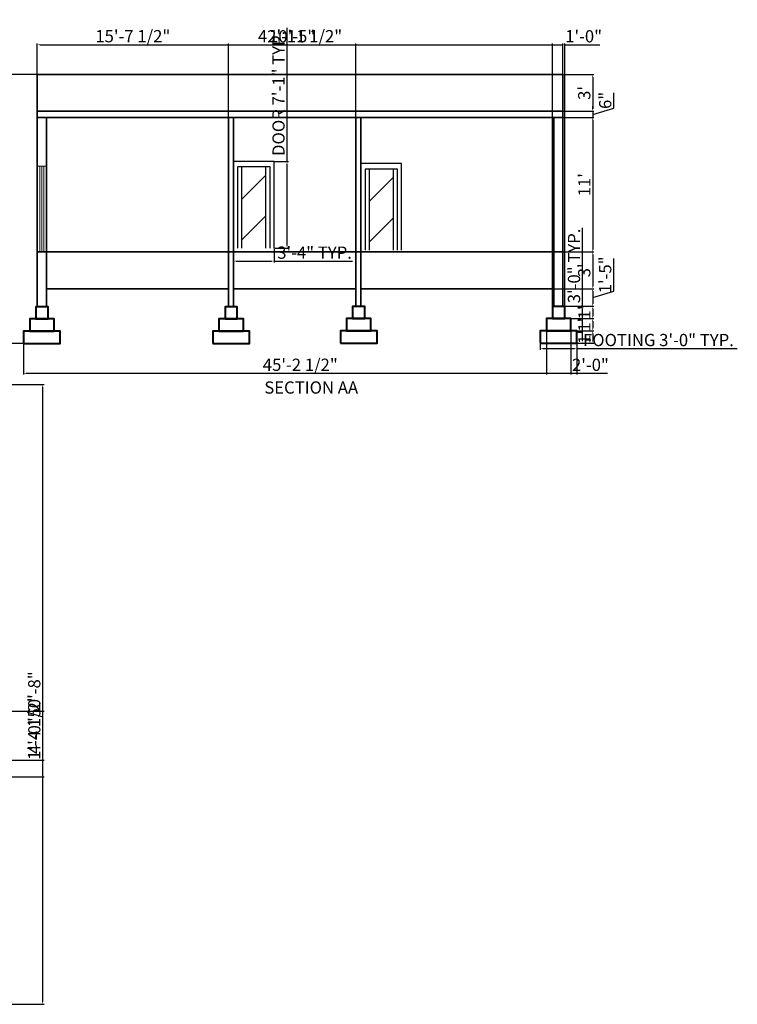
# Model space of a CAD drawing. Units: inches. Extents: x 2319 to 3765, y 2872 to 3950.
# Tile 9 of 9: x 3061 to 3765, y 2961 to 3926. Entities that reach past the tile are written whole.
import ezdxf

# ---------------------------------------------------------------- set-up
doc = ezdxf.new("R2010")
doc.units = ezdxf.units.IN
for name, color, linetype, lineweight in [('A-ANNO-DIMS', 2, 'Continuous', 18), ('A-ANNO-TEXT', 7, 'Continuous', 25), ('A-DOOR', 3, 'Continuous', 25), ('A-GLAZ', 4, 'Continuous', 18), ('A-ROOF', 7, 'Continuous', 35), ('A-SECT', 7, 'Continuous', 35), ('S-FNDN', 1, 'Continuous', 40)]:
    doc.layers.add(name, color=color, linetype=linetype, lineweight=lineweight)
doc.styles.get("Standard").update_dxf_attribs({"font": 'arial.ttf'})
doc.dimstyles.new('ISO-25', dxfattribs={"dimtxt": 12, "dimasz": 2.5, "dimexe": 1.25, "dimexo": 0.625, "dimtad": 1, "dimdec": 0, "dimlunit": 3, "dimtxsty": 'Standard', "dimcen": 2.5, "dimadec": 0, "dimazin": 0, "dimtfac": 1, "dimtdec": 0, "dimtmove": 0, "dimatfit": 3, "dimfxl": 1, "dimarcsym": 0})

# ---------------------------------------------------------------- blocks, each defined once
blk = doc.blocks.new('A$C66980853')
for p, q in [((0, 2134), (0, 0)), ((1000, 2134), (0, 2134)), ((100, 2000), (100, 0)), ((900, 2000), (100, 2000)), ((200, 2000), (200, 0)), ((800, 0), (800, 2000)), ((900, 0), (900, 2000)), ((1000, 0), (1000, 2134)), ((800, 1800), (200, 1200)), ((200, 200), (800, 800))]:
    blk.add_line(p, q)
blk = doc.blocks.new('*D31')
at = {"layer": 'A-ANNO-DIMS', "color": 0, "lineweight": -2, "transparency": 16777216}
for p, q in [((3594.69, 3872.56), (3624.59, 3872.56)), ((3623.34, 3870.06), (3623.34, 3839.06)), ((3594.69, 3836.56), (3624.59, 3836.56))]:
    blk.add_line(p, q, dxfattribs=at)
at = {"layer": 'A-ANNO-DIMS', "color": 0, "transparency": 16777216}
for points in [[(3622.92, 3870.06), (3623.75, 3870.06), (3623.34, 3872.56)], [(3622.92, 3839.06), (3623.75, 3839.06), (3623.34, 3836.56)]]:
    blk.add_solid(points, dxfattribs=at)
at = {"layer": 'Defpoints', "color": 0, "transparency": 16777216}
for p in [(3594.07, 3872.56), (3594.07, 3836.56), (3623.34, 3836.56)]:
    blk.add_point(p, dxfattribs=at)
at = {"layer": 'A-ANNO-DIMS', "color": 0, "transparency": 16777216, "insert": (3616.58, 3854.56), "char_height": 12, "attachment_point": 5, "rotation": 90}
blk.add_mtext("3'", dxfattribs=at)
blk = doc.blocks.new('*D32')
at = {"layer": 'A-ANNO-DIMS', "color": 0, "lineweight": -2, "transparency": 16777216}
for p, q in [((3643.9, 3839.73), (3643.9, 3854.84)), ((3594.69, 3836.56), (3624.59, 3836.56)), ((3623.34, 3839.06), (3623.34, 3841.56)), ((3623.34, 3833.56), (3643.9, 3839.73)), ((3623.34, 3836.56), (3623.34, 3830.56)), ((3623.34, 3836.56), (3623.34, 3830.56)), ((3594.69, 3830.56), (3624.59, 3830.56)), ((3623.34, 3828.06), (3623.34, 3825.56))]:
    blk.add_line(p, q, dxfattribs=at)
at = {"layer": 'A-ANNO-DIMS', "color": 0, "transparency": 16777216}
for points in [[(3622.92, 3839.06), (3623.75, 3839.06), (3623.34, 3836.56)], [(3622.92, 3828.06), (3623.75, 3828.06), (3623.34, 3830.56)]]:
    blk.add_solid(points, dxfattribs=at)
at = {"layer": 'Defpoints', "color": 0, "transparency": 16777216}
for p in [(3594.07, 3836.56), (3594.07, 3830.56), (3623.34, 3830.56)]:
    blk.add_point(p, dxfattribs=at)
at = {"layer": 'A-ANNO-DIMS', "color": 0, "transparency": 16777216, "insert": (3637.15, 3847.29), "char_height": 12, "attachment_point": 5, "rotation": 90}
blk.add_mtext('6"', dxfattribs=at)
blk = doc.blocks.new('*D33')
at = {"layer": 'A-ANNO-DIMS', "color": 0, "lineweight": -2, "transparency": 16777216}
for p, q in [((3594.69, 3830.56), (3624.59, 3830.56)), ((3623.34, 3828.06), (3623.34, 3701.06)), ((3594.69, 3698.56), (3624.59, 3698.56))]:
    blk.add_line(p, q, dxfattribs=at)
at = {"layer": 'A-ANNO-DIMS', "color": 0, "transparency": 16777216}
for points in [[(3622.92, 3828.06), (3623.75, 3828.06), (3623.34, 3830.56)], [(3622.92, 3701.06), (3623.75, 3701.06), (3623.34, 3698.56)]]:
    blk.add_solid(points, dxfattribs=at)
at = {"layer": 'Defpoints', "color": 0, "transparency": 16777216}
for p in [(3594.07, 3830.56), (3594.07, 3698.56), (3623.34, 3698.56)]:
    blk.add_point(p, dxfattribs=at)
at = {"layer": 'A-ANNO-DIMS', "color": 0, "transparency": 16777216, "insert": (3616.69, 3764.56), "char_height": 12, "attachment_point": 5, "rotation": 90}
blk.add_mtext("11'", dxfattribs=at)
blk = doc.blocks.new('*D34')
at = {"layer": 'A-ANNO-DIMS', "color": 0, "lineweight": -2, "transparency": 16777216}
for p, q in [((3594.69, 3698.56), (3624.59, 3698.56)), ((3623.34, 3696.06), (3623.34, 3665.06)), ((3585.69, 3662.56), (3624.59, 3662.56))]:
    blk.add_line(p, q, dxfattribs=at)
at = {"layer": 'A-ANNO-DIMS', "color": 0, "transparency": 16777216}
for points in [[(3622.92, 3696.06), (3623.75, 3696.06), (3623.34, 3698.56)], [(3622.92, 3665.06), (3623.75, 3665.06), (3623.34, 3662.56)]]:
    blk.add_solid(points, dxfattribs=at)
at = {"layer": 'Defpoints', "color": 0, "transparency": 16777216}
for p in [(3594.07, 3698.56), (3585.07, 3662.56), (3623.34, 3662.56)]:
    blk.add_point(p, dxfattribs=at)
at = {"layer": 'A-ANNO-DIMS', "color": 0, "transparency": 16777216, "insert": (3616.58, 3680.56), "char_height": 12, "attachment_point": 5, "rotation": 90}
blk.add_mtext("3'", dxfattribs=at)
blk = doc.blocks.new('*D35')
at = {"layer": 'A-ANNO-DIMS', "color": 0, "lineweight": -2, "transparency": 16777216}
for p, q in [((3643.9, 3660.13), (3643.9, 3692.15)), ((3585.69, 3662.56), (3624.59, 3662.56)), ((3623.34, 3653.96), (3643.9, 3660.13)), ((3623.34, 3660.06), (3623.34, 3647.85)), ((3594.69, 3645.35), (3624.59, 3645.35))]:
    blk.add_line(p, q, dxfattribs=at)
at = {"layer": 'A-ANNO-DIMS', "color": 0, "transparency": 16777216}
for points in [[(3622.92, 3660.06), (3623.75, 3660.06), (3623.34, 3662.56)], [(3622.92, 3647.85), (3623.75, 3647.85), (3623.34, 3645.35)]]:
    blk.add_solid(points, dxfattribs=at)
at = {"layer": 'Defpoints', "color": 0, "transparency": 16777216}
for p in [(3585.07, 3662.56), (3594.07, 3645.35), (3623.34, 3645.35)]:
    blk.add_point(p, dxfattribs=at)
at = {"layer": 'A-ANNO-DIMS', "color": 0, "transparency": 16777216, "insert": (3637.15, 3676.14), "char_height": 12, "attachment_point": 5, "rotation": 90}
blk.add_mtext('1\'-5"', dxfattribs=at)
blk = doc.blocks.new('*D36')
at = {"layer": 'A-ANNO-DIMS', "color": 0, "lineweight": -2, "transparency": 16777216}
for p, q in [((3594.69, 3645.35), (3624.59, 3645.35)), ((3623.34, 3642.85), (3623.34, 3635.72)), ((3596.53, 3633.22), (3624.59, 3633.22))]:
    blk.add_line(p, q, dxfattribs=at)
at = {"layer": 'A-ANNO-DIMS', "color": 0, "transparency": 16777216}
for points in [[(3622.92, 3642.85), (3623.75, 3642.85), (3623.34, 3645.35)], [(3622.92, 3635.72), (3623.75, 3635.72), (3623.34, 3633.22)]]:
    blk.add_solid(points, dxfattribs=at)
at = {"layer": 'Defpoints', "color": 0, "transparency": 16777216}
for p in [(3594.07, 3645.35), (3595.91, 3633.22), (3623.34, 3633.22)]:
    blk.add_point(p, dxfattribs=at)
at = {"layer": 'A-ANNO-DIMS', "color": 0, "transparency": 16777216, "insert": (3616.69, 3639.28), "char_height": 12, "attachment_point": 5, "rotation": 90}
blk.add_mtext("1'", dxfattribs=at)
blk = doc.blocks.new('*D37')
at = {"layer": 'A-ANNO-DIMS', "color": 0, "lineweight": -2, "transparency": 16777216}
for p, q in [((3596.53, 3633.22), (3624.59, 3633.22)), ((3623.34, 3630.72), (3623.34, 3623.72)), ((3602.53, 3621.22), (3624.59, 3621.22))]:
    blk.add_line(p, q, dxfattribs=at)
at = {"layer": 'A-ANNO-DIMS', "color": 0, "transparency": 16777216}
for points in [[(3622.92, 3630.72), (3623.75, 3630.72), (3623.34, 3633.22)], [(3622.92, 3623.72), (3623.75, 3623.72), (3623.34, 3621.22)]]:
    blk.add_solid(points, dxfattribs=at)
at = {"layer": 'Defpoints', "color": 0, "transparency": 16777216}
for p in [(3595.91, 3633.22), (3601.91, 3621.22), (3623.34, 3621.22)]:
    blk.add_point(p, dxfattribs=at)
at = {"layer": 'A-ANNO-DIMS', "color": 0, "transparency": 16777216, "insert": (3616.69, 3627.22), "char_height": 12, "attachment_point": 5, "rotation": 90}
blk.add_mtext("1'", dxfattribs=at)
blk = doc.blocks.new('*D38')
at = {"layer": 'A-ANNO-DIMS', "color": 0, "lineweight": -2, "transparency": 16777216}
for p, q in [((3602.53, 3621.22), (3624.59, 3621.22)), ((3623.34, 3618.72), (3623.34, 3611.72)), ((3608.53, 3609.22), (3624.59, 3609.22))]:
    blk.add_line(p, q, dxfattribs=at)
at = {"layer": 'A-ANNO-DIMS', "color": 0, "transparency": 16777216}
for points in [[(3622.92, 3618.72), (3623.75, 3618.72), (3623.34, 3621.22)], [(3622.92, 3611.72), (3623.75, 3611.72), (3623.34, 3609.22)]]:
    blk.add_solid(points, dxfattribs=at)
at = {"layer": 'Defpoints', "color": 0, "transparency": 16777216}
for p in [(3601.91, 3621.22), (3607.91, 3609.22), (3623.34, 3609.22)]:
    blk.add_point(p, dxfattribs=at)
at = {"layer": 'A-ANNO-DIMS', "color": 0, "transparency": 16777216, "insert": (3616.69, 3615.22), "char_height": 12, "attachment_point": 5, "rotation": 90}
blk.add_mtext("1'", dxfattribs=at)
blk = doc.blocks.new('FOOTING-36-STEPPED-SECT')
for points in [[(12, 24), (24, 24), (24, 36), (12, 36)], [(6, 12), (30, 12), (30, 24), (6, 24)], [(0, 0), (36, 0), (36, 12), (0, 12)]]:
    blk.add_lwpolyline(points, close=True)
blk = doc.blocks.new('*D65')
at = {"layer": 'A-ANNO-DIMS', "color": 0, "lineweight": -2, "transparency": 16777216}
for p, q in [((3323.59, 3787.27), (3323.59, 3918.52)), ((3311.48, 3787.27), (3324.84, 3787.27)), ((3323.59, 3704.85), (3323.59, 3784.77)), ((3311.48, 3702.35), (3324.84, 3702.35))]:
    blk.add_line(p, q, dxfattribs=at)
at = {"layer": 'A-ANNO-DIMS', "color": 0, "transparency": 16777216}
for points in [[(3323.18, 3784.77), (3324.01, 3784.77), (3323.59, 3787.27)], [(3323.18, 3704.85), (3324.01, 3704.85), (3323.59, 3702.35)]]:
    blk.add_solid(points, dxfattribs=at)
at = {"layer": 'Defpoints', "color": 0, "transparency": 16777216}
for p in [(3310.86, 3787.27), (3323.59, 3787.27), (3310.86, 3702.35)]:
    blk.add_point(p, dxfattribs=at)
at = {"layer": 'A-ANNO-DIMS', "color": 0, "transparency": 16777216, "insert": (3316.76, 3854.14), "char_height": 12, "attachment_point": 5, "rotation": 90}
blk.add_mtext('DOOR 7\'-1" TYP.', dxfattribs=at)
blk = doc.blocks.new('*D66')
at = {"layer": 'A-ANNO-DIMS', "color": 0, "lineweight": -2, "transparency": 16777216}
for p, q in [((3271.07, 3701.73), (3271.07, 3688.36)), ((3310.86, 3701.73), (3310.86, 3688.36)), ((3273.57, 3689.61), (3308.36, 3689.61)), ((3310.86, 3689.61), (3387.74, 3689.61))]:
    blk.add_line(p, q, dxfattribs=at)
at = {"layer": 'A-ANNO-DIMS', "color": 0, "transparency": 16777216}
for points in [[(3273.57, 3690.03), (3273.57, 3689.2), (3271.07, 3689.61)], [(3308.36, 3690.03), (3308.36, 3689.2), (3310.86, 3689.61)]]:
    blk.add_solid(points, dxfattribs=at)
at = {"layer": 'Defpoints', "color": 0, "transparency": 16777216}
for p in [(3271.07, 3702.35), (3310.86, 3702.35), (3310.86, 3689.61)]:
    blk.add_point(p, dxfattribs=at)
at = {"layer": 'A-ANNO-DIMS', "color": 0, "transparency": 16777216, "insert": (3350.55, 3696.37), "char_height": 12, "attachment_point": 5}
blk.add_mtext('3\'-4" TYP.', dxfattribs=at)
blk = doc.blocks.new('*D69')
at = {"layer": 'A-ANNO-DIMS', "color": 0, "lineweight": -2, "transparency": 16777216}
for p, q in [((3571.91, 3608.59), (3571.91, 3602.57)), ((3574.41, 3603.82), (3605.41, 3603.82)), ((3607.91, 3608.59), (3607.91, 3602.57)), ((3607.91, 3603.82), (3765.15, 3603.82))]:
    blk.add_line(p, q, dxfattribs=at)
at = {"layer": 'A-ANNO-DIMS', "color": 0, "transparency": 16777216}
for points in [[(3574.41, 3604.23), (3574.41, 3603.4), (3571.91, 3603.82)], [(3605.41, 3604.23), (3605.41, 3603.4), (3607.91, 3603.82)]]:
    blk.add_solid(points, dxfattribs=at)
at = {"layer": 'Defpoints', "color": 0, "transparency": 16777216}
for p in [(3571.91, 3609.22), (3607.91, 3609.22), (3607.91, 3603.82)]:
    blk.add_point(p, dxfattribs=at)
at = {"layer": 'A-ANNO-DIMS', "color": 0, "transparency": 16777216, "insert": (3687.78, 3610.65), "char_height": 12, "attachment_point": 5}
blk.add_mtext('FOOTING 3\'-0" TYP.', dxfattribs=at)
blk = doc.blocks.new('*D70')
at = {"layer": 'A-ANNO-DIMS', "color": 0, "lineweight": -2, "transparency": 16777216}
for p, q in [((3613.31, 3645.22), (3613.31, 3722.1)), ((3608.53, 3645.22), (3614.56, 3645.22)), ((3613.31, 3611.72), (3613.31, 3642.72)), ((3608.53, 3609.22), (3614.56, 3609.22))]:
    blk.add_line(p, q, dxfattribs=at)
at = {"layer": 'A-ANNO-DIMS', "color": 0, "transparency": 16777216}
for points in [[(3612.89, 3642.72), (3613.73, 3642.72), (3613.31, 3645.22)], [(3612.89, 3611.72), (3613.73, 3611.72), (3613.31, 3609.22)]]:
    blk.add_solid(points, dxfattribs=at)
at = {"layer": 'Defpoints', "color": 0, "transparency": 16777216}
for p in [(3607.91, 3645.22), (3613.31, 3645.22), (3607.91, 3609.22)]:
    blk.add_point(p, dxfattribs=at)
at = {"layer": 'A-ANNO-DIMS', "color": 0, "transparency": 16777216, "insert": (3606.55, 3684.91), "char_height": 12, "attachment_point": 5, "rotation": 90}
blk.add_mtext('3\'-0" TYP.', dxfattribs=at)
blk = doc.blocks.new('*D72')
at = {"layer": 'A-ANNO-DIMS', "color": 0, "lineweight": -2, "transparency": 16777216}
for p, q in [((2955.75, 3568.61), (3085.2, 3568.61)), ((3083.95, 2963.11), (3083.95, 3566.11)), ((2955.75, 2960.61), (3085.2, 2960.61))]:
    blk.add_line(p, q, dxfattribs=at)
at = {"layer": 'A-ANNO-DIMS', "color": 0, "transparency": 16777216}
for points in [[(3083.53, 3566.11), (3084.36, 3566.11), (3083.95, 3568.61)], [(3083.53, 2963.11), (3084.36, 2963.11), (3083.95, 2960.61)]]:
    blk.add_solid(points, dxfattribs=at)
at = {"layer": 'Defpoints', "color": 0, "transparency": 16777216}
for p in [(2955.13, 3568.61), (3083.95, 3568.61), (2955.13, 2960.61)]:
    blk.add_point(p, dxfattribs=at)
at = {"layer": 'A-ANNO-DIMS', "color": 0, "transparency": 16777216, "insert": (3077.2, 3264.61), "char_height": 12, "attachment_point": 5, "rotation": 90}
blk.add_mtext('50\'-8"', dxfattribs=at)
blk = doc.blocks.new('*D81')
at = {"layer": 'A-ANNO-DIMS', "color": 0, "lineweight": -2, "transparency": 16777216}
for p, q in [((2603.75, 3248.11), (3085.2, 3248.11)), ((3083.95, 3202.61), (3083.95, 3245.61)), ((2603.75, 3200.11), (3085.2, 3200.11))]:
    blk.add_line(p, q, dxfattribs=at)
at = {"layer": 'A-ANNO-DIMS', "color": 0, "transparency": 16777216}
for points in [[(3083.53, 3245.61), (3084.36, 3245.61), (3083.95, 3248.11)], [(3083.53, 3202.61), (3084.36, 3202.61), (3083.95, 3200.11)]]:
    blk.add_solid(points, dxfattribs=at)
at = {"layer": 'Defpoints', "color": 0, "transparency": 16777216}
for p in [(2603.13, 3248.11), (3083.95, 3248.11), (2603.13, 3200.11)]:
    blk.add_point(p, dxfattribs=at)
at = {"layer": 'A-ANNO-DIMS', "color": 0, "transparency": 16777216, "insert": (3077.2, 3224.11), "char_height": 12, "attachment_point": 5, "rotation": 90}
blk.add_mtext('4\'-0"', dxfattribs=at)
blk = doc.blocks.new('*D82')
at = {"layer": 'A-ANNO-DIMS', "color": 0, "lineweight": -2, "transparency": 16777216}
for p, q in [((3083.95, 3200.11), (3083.95, 3262.59)), ((2603.75, 3200.11), (3085.2, 3200.11)), ((3083.95, 3186.11), (3083.95, 3197.61)), ((2603.75, 3183.61), (3085.2, 3183.61))]:
    blk.add_line(p, q, dxfattribs=at)
at = {"layer": 'A-ANNO-DIMS', "color": 0, "transparency": 16777216}
for points in [[(3083.53, 3197.61), (3084.36, 3197.61), (3083.95, 3200.11)], [(3083.53, 3186.11), (3084.36, 3186.11), (3083.95, 3183.61)]]:
    blk.add_solid(points, dxfattribs=at)
at = {"layer": 'Defpoints', "color": 0, "transparency": 16777216}
for p in [(2603.13, 3200.11), (3083.95, 3200.11), (2603.13, 3183.61)]:
    blk.add_point(p, dxfattribs=at)
at = {"layer": 'A-ANNO-DIMS', "color": 0, "transparency": 16777216, "insert": (3077.12, 3232.6), "char_height": 12, "attachment_point": 5, "rotation": 90}
blk.add_mtext('1\'-4 1/2"', dxfattribs=at)
blk = doc.blocks.new('*D96')
at = {"layer": 'A-ANNO-DIMS', "color": 0, "lineweight": -2, "transparency": 16777216}
for p, q in [((3065.2, 3608.23), (3065.2, 3578.31)), ((3607.91, 3608.59), (3607.91, 3578.31)), ((3067.7, 3579.56), (3605.41, 3579.56))]:
    blk.add_line(p, q, dxfattribs=at)
at = {"layer": 'A-ANNO-DIMS', "color": 0, "transparency": 16777216}
for points in [[(3067.7, 3579.97), (3067.7, 3579.14), (3065.2, 3579.56)], [(3605.41, 3579.97), (3605.41, 3579.14), (3607.91, 3579.56)]]:
    blk.add_solid(points, dxfattribs=at)
at = {"layer": 'Defpoints', "color": 0, "transparency": 16777216}
for p in [(3065.2, 3608.86), (3607.91, 3609.22), (3607.91, 3579.56)]:
    blk.add_point(p, dxfattribs=at)
at = {"layer": 'A-ANNO-DIMS', "color": 0, "transparency": 16777216, "insert": (3336.55, 3586.39), "char_height": 12, "attachment_point": 5}
blk.add_mtext('45\'-2 1/2"', dxfattribs=at)
blk = doc.blocks.new('*D97')
at = {"layer": 'A-ANNO-DIMS', "color": 0, "lineweight": -2, "transparency": 16777216}
for p, q in [((3077.94, 3872.56), (3034.65, 3872.56)), ((3035.9, 3611.36), (3035.9, 3870.06)), ((3064.57, 3608.86), (3034.65, 3608.86))]:
    blk.add_line(p, q, dxfattribs=at)
at = {"layer": 'A-ANNO-DIMS', "color": 0, "transparency": 16777216}
for points in [[(3035.48, 3870.06), (3036.31, 3870.06), (3035.9, 3872.56)], [(3035.48, 3611.36), (3036.31, 3611.36), (3035.9, 3608.86)]]:
    blk.add_solid(points, dxfattribs=at)
at = {"layer": 'Defpoints', "color": 0, "transparency": 16777216}
for p in [(3035.9, 3872.56), (3078.57, 3872.56), (3065.2, 3608.86)]:
    blk.add_point(p, dxfattribs=at)
at = {"layer": 'A-ANNO-DIMS', "color": 0, "transparency": 16777216, "insert": (3029.07, 3740.71), "char_height": 12, "attachment_point": 5, "rotation": 90}
blk.add_mtext('21\'-11 1/2"', dxfattribs=at)
blk = doc.blocks.new('*D98')
at = {"layer": 'A-ANNO-DIMS', "color": 0, "lineweight": -2, "transparency": 16777216}
for p, q in [((3078.57, 3873.19), (3078.57, 3903.11)), ((3594.07, 3873.19), (3594.07, 3903.11)), ((3081.07, 3901.86), (3591.57, 3901.86))]:
    blk.add_line(p, q, dxfattribs=at)
at = {"layer": 'A-ANNO-DIMS', "color": 0, "transparency": 16777216}
for points in [[(3081.07, 3902.28), (3081.07, 3901.44), (3078.57, 3901.86)], [(3591.57, 3902.28), (3591.57, 3901.44), (3594.07, 3901.86)]]:
    blk.add_solid(points, dxfattribs=at)
at = {"layer": 'Defpoints', "color": 0, "transparency": 16777216}
for p in [(3594.07, 3901.86), (3078.57, 3872.56), (3594.07, 3872.56)]:
    blk.add_point(p, dxfattribs=at)
at = {"layer": 'A-ANNO-DIMS', "color": 0, "transparency": 16777216, "insert": (3336.32, 3908.69), "char_height": 12, "attachment_point": 5}
blk.add_mtext('42\'-11 1/2"', dxfattribs=at)
blk = doc.blocks.new('*D99')
at = {"layer": 'A-ANNO-DIMS', "color": 0, "lineweight": -2, "transparency": 16777216}
for p, q in [((3078.57, 3831.19), (3078.57, 3903.11)), ((3266.07, 3831.19), (3266.07, 3903.11)), ((3081.07, 3901.86), (3263.57, 3901.86))]:
    blk.add_line(p, q, dxfattribs=at)
at = {"layer": 'A-ANNO-DIMS', "color": 0, "transparency": 16777216}
for points in [[(3081.07, 3902.28), (3081.07, 3901.44), (3078.57, 3901.86)], [(3263.57, 3902.28), (3263.57, 3901.44), (3266.07, 3901.86)]]:
    blk.add_solid(points, dxfattribs=at)
at = {"layer": 'Defpoints', "color": 0, "transparency": 16777216}
for p in [(3266.07, 3901.86), (3078.57, 3830.56), (3266.07, 3830.56)]:
    blk.add_point(p, dxfattribs=at)
at = {"layer": 'A-ANNO-DIMS', "color": 0, "transparency": 16777216, "insert": (3172.32, 3908.69), "char_height": 12, "attachment_point": 5}
blk.add_mtext('15\'-7 1/2"', dxfattribs=at)
blk = doc.blocks.new('*D100')
at = {"layer": 'A-ANNO-DIMS', "color": 0, "lineweight": -2, "transparency": 16777216}
for p, q in [((3266.07, 3831.19), (3266.07, 3903.11)), ((3391.07, 3831.19), (3391.07, 3903.11)), ((3268.57, 3901.86), (3388.57, 3901.86))]:
    blk.add_line(p, q, dxfattribs=at)
at = {"layer": 'A-ANNO-DIMS', "color": 0, "transparency": 16777216}
for points in [[(3268.57, 3902.28), (3268.57, 3901.44), (3266.07, 3901.86)], [(3388.57, 3902.28), (3388.57, 3901.44), (3391.07, 3901.86)]]:
    blk.add_solid(points, dxfattribs=at)
at = {"layer": 'Defpoints', "color": 0, "transparency": 16777216}
for p in [(3391.07, 3901.86), (3266.07, 3830.56), (3391.07, 3830.56)]:
    blk.add_point(p, dxfattribs=at)
at = {"layer": 'A-ANNO-DIMS', "color": 0, "transparency": 16777216, "insert": (3328.57, 3908.61), "char_height": 12, "attachment_point": 5}
blk.add_mtext('10\'-5"', dxfattribs=at)
blk = doc.blocks.new('*D101')
at = {"layer": 'A-ANNO-DIMS', "color": 0, "lineweight": -2, "transparency": 16777216}
for p, q in [((3577.91, 3632.59), (3577.91, 3578.31)), ((3601.91, 3632.59), (3601.91, 3578.31)), ((3580.41, 3579.56), (3599.41, 3579.56)), ((3601.91, 3579.56), (3637.76, 3579.56))]:
    blk.add_line(p, q, dxfattribs=at)
at = {"layer": 'A-ANNO-DIMS', "color": 0, "transparency": 16777216}
for points in [[(3580.41, 3579.97), (3580.41, 3579.14), (3577.91, 3579.56)], [(3599.41, 3579.97), (3599.41, 3579.14), (3601.91, 3579.56)]]:
    blk.add_solid(points, dxfattribs=at)
at = {"layer": 'Defpoints', "color": 0, "transparency": 16777216}
for p in [(3577.91, 3633.22), (3601.91, 3633.22), (3601.91, 3579.56)]:
    blk.add_point(p, dxfattribs=at)
at = {"layer": 'A-ANNO-DIMS', "color": 0, "transparency": 16777216, "insert": (3621.09, 3586.31), "char_height": 12, "attachment_point": 5}
blk.add_mtext('2\'-0"', dxfattribs=at)
blk = doc.blocks.new('*D102')
at = {"layer": 'A-ANNO-DIMS', "color": 0, "lineweight": -2, "transparency": 16777216}
for p, q in [((3583.91, 3645.84), (3583.91, 3903.11)), ((3595.91, 3645.84), (3595.91, 3903.11)), ((3586.41, 3901.86), (3593.41, 3901.86)), ((3595.91, 3901.86), (3630.43, 3901.86))]:
    blk.add_line(p, q, dxfattribs=at)
at = {"layer": 'A-ANNO-DIMS', "color": 0, "transparency": 16777216}
for points in [[(3586.41, 3902.28), (3586.41, 3901.44), (3583.91, 3901.86)], [(3593.41, 3902.28), (3593.41, 3901.44), (3595.91, 3901.86)]]:
    blk.add_solid(points, dxfattribs=at)
at = {"layer": 'Defpoints', "color": 0, "transparency": 16777216}
for p in [(3595.91, 3901.86), (3583.91, 3645.22), (3595.91, 3645.22)]:
    blk.add_point(p, dxfattribs=at)
at = {"layer": 'A-ANNO-DIMS', "color": 0, "transparency": 16777216, "insert": (3614.42, 3908.61), "char_height": 12, "attachment_point": 5}
blk.add_mtext('1\'-0"', dxfattribs=at)

msp = doc.modelspace()

# ---------------------------------------------------------------- linework, layer by layer
at = {"layer": 'A-GLAZ'}
for p, q in [((3078.57, 3782.64), (3087.57, 3782.64)), ((3081.07, 3782.64), (3081.07, 3698.64)), ((3083.07, 3782.64), (3083.07, 3698.64)), ((3085.07, 3782.64), (3085.07, 3698.64))]:
    msp.add_line(p, q, dxfattribs=at)
at = {"layer": 'A-ROOF'}
for p, q in [((3078.57, 3872.56), (3594.07, 3872.56)), ((3078.57, 3836.56), (3594.07, 3836.56)), ((3078.57, 3830.56), (3594.07, 3830.56))]:
    msp.add_line(p, q, dxfattribs=at)
at = {"layer": 'A-SECT'}
for p, q in [((3078.57, 3645.35), (3078.57, 3872.56)), ((3594.07, 3645.35), (3594.07, 3872.56)), ((3087.57, 3645.54), (3087.57, 3830.56)), ((3266.07, 3645.35), (3266.07, 3830.56)), ((3271.07, 3645.35), (3271.07, 3830.56)), ((3391.07, 3645.35), (3391.07, 3830.56)), ((3396.07, 3645.35), (3396.07, 3830.56)), ((3585.07, 3645.35), (3585.07, 3830.56)), ((3078.57, 3698.56), (3594.07, 3698.56)), ((3087.57, 3662.56), (3266.07, 3662.56)), ((3271.07, 3662.56), (3391.07, 3662.56)), ((3396.07, 3662.56), (3585.07, 3662.56))]:
    msp.add_line(p, q, dxfattribs=at)

# ---------------------------------------------------------------- block references
at = {"layer": 'A-DOOR', "xscale": 0.0397894998909496, "yscale": 0.0397894998909496, "zscale": 0.0397894998909496}
for p in [(3271.07, 3702.35), (3396.07, 3700.31)]:
    msp.add_blockref('A$C66980853', p, dxfattribs=at)
at = {"layer": 'S-FNDN'}
for p in [(3065.2, 3608.86), (3250.78, 3608.86), (3375.88, 3609.21), (3571.91, 3609.22)]:
    msp.add_blockref('FOOTING-36-STEPPED-SECT', p, dxfattribs=at)

# ---------------------------------------------------------------- texts
at = {"layer": 'A-ANNO-TEXT'}
msp.add_text('SECTION AA', height=12, dxfattribs=at).set_placement((3301.25, 3559.62))

# ---------------------------------------------------------------- dimensions: what is measured, and where the dimension line sits
at = {"layer": 'A-ANNO-DIMS'}
for base, p1, p2, picture, middle in [((3594.07, 3901.86), (3078.57, 3872.56), (3594.07, 3872.56), '*D98', (3336.32, 3908.69)), ((3266.07, 3901.86), (3078.57, 3830.56), (3266.07, 3830.56), '*D99', (3172.32, 3908.69)), ((3391.07, 3901.86), (3266.07, 3830.56), (3391.07, 3830.56), '*D100', (3328.57, 3908.61)), ((3595.91, 3901.86), (3583.91, 3645.22), (3595.91, 3645.22), '*D102', (3614.42, 3908.61)), ((3601.91, 3579.56), (3577.91, 3633.22), (3601.91, 3633.22), '*D101', (3621.09, 3586.31)), ((3607.91, 3579.56), (3065.2, 3608.86), (3607.91, 3609.22), '*D96', (3336.55, 3586.39))]:
    dim = msp.add_linear_dim(base=base, p1=p1, p2=p2, dimstyle='ISO-25', override={"dimdec": 1, "dimlfac": 1, "dimrnd": 0, "dimzin": 1, "dimdsep": 46, "dimlunit": 4, "dimfrac": 2}, dxfattribs=at)
    dim.commit()
    dim.dimension.update_dxf_attribs({"geometry": picture, "text_midpoint": middle})
for base, p1, p2, text, picture, middle in [((3323.59, 3787.27), (3310.86, 3702.35), (3310.86, 3787.27), 'DOOR <> TYP.', '*D65', (3316.76, 3854.14)), ((3613.31, 3645.22), (3607.91, 3609.22), (3607.91, 3645.22), '<> TYP.', '*D70', (3606.55, 3684.91))]:
    dim = msp.add_linear_dim(base=base, p1=p1, p2=p2, angle=90, text=text, dimstyle='ISO-25', override={"dimdec": 1, "dimlfac": 1, "dimrnd": 0, "dimzin": 1, "dimdsep": 46, "dimlunit": 4, "dimfrac": 2}, dxfattribs=at)
    dim.commit()
    dim.dimension.update_dxf_attribs({"geometry": picture, "text_midpoint": middle})
for base, p1, p2, override, picture, middle in [((3035.9, 3872.56), (3065.2, 3608.86), (3078.57, 3872.56), {"dimdec": 1, "dimlfac": 1, "dimrnd": 0, "dimzin": 1, "dimdsep": 46, "dimlunit": 4, "dimfrac": 2}, '*D97', (3029.07, 3740.71)), ((3623.34, 3836.56), (3594.07, 3872.56), (3594.07, 3836.56), {"dimclrd": 0, "dimclre": 0, "dimclrt": 0}, '*D31', (3616.58, 3854.56)), ((3623.34, 3830.56), (3594.07, 3836.56), (3594.07, 3830.56), {"dimclrd": 0, "dimclre": 0, "dimclrt": 0, "dimtmove": 1}, '*D32', (3637.15, 3840.36)), ((3623.34, 3698.56), (3594.07, 3830.56), (3594.07, 3698.56), {"dimclrd": 0, "dimclre": 0, "dimclrt": 0, "dimtmove": 1}, '*D33', (3616.69, 3764.56)), ((3623.34, 3662.56), (3594.07, 3698.56), (3585.07, 3662.56), {"dimclrd": 0, "dimclre": 0, "dimclrt": 0, "dimtmove": 1}, '*D34', (3616.58, 3680.56)), ((3623.34, 3645.35), (3585.07, 3662.56), (3594.07, 3645.35), {"dimclrd": 0, "dimclre": 0, "dimclrt": 0, "dimtmove": 1}, '*D35', (3637.15, 3660.75)), ((3623.34, 3633.22), (3594.07, 3645.35), (3595.91, 3633.22), {"dimclrd": 0, "dimclre": 0, "dimclrt": 0, "dimtmove": 1}, '*D36', (3616.69, 3639.28)), ((3623.34, 3621.22), (3595.91, 3633.22), (3601.91, 3621.22), {"dimclrd": 0, "dimclre": 0, "dimclrt": 0, "dimtmove": 1}, '*D37', (3616.69, 3627.22)), ((3623.34, 3609.22), (3601.91, 3621.22), (3607.91, 3609.22), {"dimclrd": 0, "dimclre": 0, "dimclrt": 0, "dimtmove": 1}, '*D38', (3616.69, 3615.22)), ((3083.95, 3568.61), (2955.13, 2960.61), (2955.13, 3568.61), {"dimdec": 1, "dimlfac": 1, "dimrnd": 0, "dimzin": 1, "dimdsep": 46, "dimlunit": 4, "dimfrac": 2}, '*D72', (3077.2, 3264.61)), ((3083.95, 3200.11), (2603.13, 3183.61), (2603.13, 3200.11), {"dimdec": 1, "dimlfac": 1, "dimrnd": 0, "dimzin": 1, "dimdsep": 46, "dimlunit": 4, "dimfrac": 2}, '*D82', (3077.12, 3232.6)), ((3083.95, 3248.11), (2603.13, 3200.11), (2603.13, 3248.11), {"dimdec": 1, "dimlfac": 1, "dimrnd": 0, "dimzin": 1, "dimdsep": 46, "dimlunit": 4, "dimfrac": 2}, '*D81', (3077.2, 3224.11))]:
    dim = msp.add_linear_dim(base=base, p1=p1, p2=p2, angle=90, dimstyle='ISO-25', override=override, dxfattribs=at)
    dim.commit()
    dim.dimension.update_dxf_attribs({"geometry": picture, "text_midpoint": middle})
for base, p1, p2, text, picture, middle in [((3310.86, 3689.61), (3271.07, 3702.35), (3310.86, 3702.35), '<> TYP.', '*D66', (3350.55, 3696.37)), ((3607.91, 3603.82), (3571.91, 3609.22), (3607.91, 3609.22), 'FOOTING <> TYP.', '*D69', (3687.78, 3610.65))]:
    dim = msp.add_linear_dim(base=base, p1=p1, p2=p2, text=text, dimstyle='ISO-25', override={"dimdec": 1, "dimlfac": 1, "dimrnd": 0, "dimzin": 1, "dimdsep": 46, "dimlunit": 4, "dimfrac": 2}, dxfattribs=at)
    dim.commit()
    dim.dimension.update_dxf_attribs({"geometry": picture, "text_midpoint": middle})

doc.saveas('drawing.dxf')
